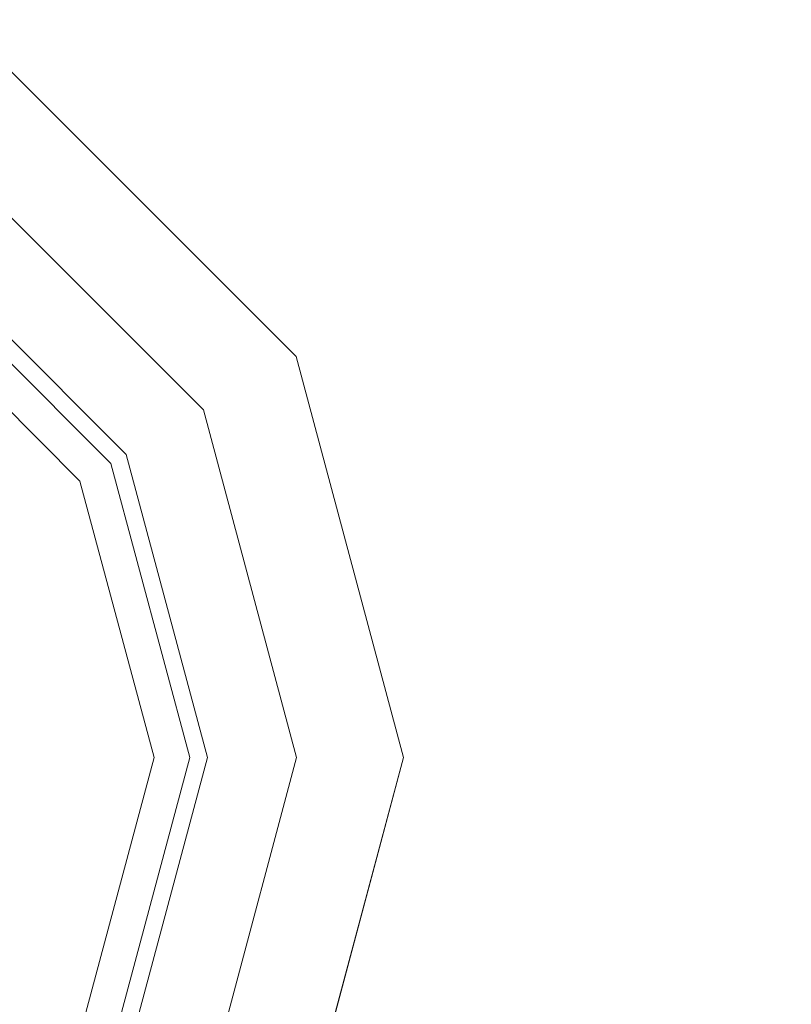
# Model space of a CAD drawing. Units: inches. Extents: x 375 to 1122, y 27 to 1069.
# Tile 123 of 155: x 715.443 to 720.771, y 893.412 to 900.211. Entities that reach past the tile are written whole.
import ezdxf

# ---------------------------------------------------------------- set-up
doc = ezdxf.new("R2010")
doc.units = ezdxf.units.IN
doc.layers.add('A-ANNO-DIMS', color=2, linetype='Continuous', lineweight=18)
doc.layers.add('Furniture', color=30, linetype='Continuous', lineweight=18)
doc.styles.get("Standard").update_dxf_attribs({"font": 'arial.ttf'})
doc.dimstyles.new('ISO-25', dxfattribs={"dimtxt": 12, "dimasz": 2.5, "dimexe": 1.5, "dimexo": 1.5, "dimtad": 1, "dimdec": 1, "dimlunit": 3, "dimtxsty": 'Standard', "dimblk": 'ARCHTICK', "dimcen": 2.5, "dimadec": 0, "dimazin": 0, "dimtfac": 1, "dimtdec": 1, "dimtmove": 0, "dimatfit": 3, "dimfxl": 1.5, "dimfxlon": 1, "dimarcsym": 0})

# ---------------------------------------------------------------- blocks, each defined once
blk = doc.blocks.new('A$C403C54AD')
at = {"linetype": 'ByBlock'}
for points, invisible_edges in [([(1.0802, 0.82864, -0.00874), (1.0802, 0.81017, -0.00874), (1.02018, 0.79408, -0.00874), (1.01094, 0.81008, -0.00874)], 5), ([(1.0802, 0.79478, -0.02259), (1.0802, 0.82864, -0.01335), (1.01094, 0.81008, -0.01335), (1.02787, 0.78075, -0.02259)], 5), ([(1.14947, 0.81008, -0.00874), (1.14023, 0.79408, -0.00874), (1.0802, 0.81017, -0.00874), (1.0802, 0.82864, -0.00874)], 5), ([(1.13254, 0.78075, -0.02259), (1.14947, 0.81008, -0.01335), (1.0802, 0.82864, -0.01335), (1.0802, 0.79478, -0.02259)], 5), ([(1.01094, 0.81008, -0.00874), (1.02018, 0.79408, -0.00874), (0.97623, 0.75014, -0.00874), (0.96024, 0.75938, -0.00874)], 5), ([(1.02787, 0.78075, -0.02259), (1.01094, 0.81008, -0.01335), (0.96024, 0.75938, -0.01335), (0.98956, 0.74244, -0.02259)], 5), ([(1.0802, 0.81017, -0.00874), (1.0802, 0.7917, -0.01489), (1.02941, 0.77809, -0.01489), (1.02018, 0.79408, -0.00874)], 5), ([(1.14023, 0.79408, -0.00874), (1.131, 0.77809, -0.01489), (1.0802, 0.7917, -0.01489), (1.0802, 0.81017, -0.00874)], 5), ([(1.02018, 0.79408, -0.00874), (1.02941, 0.77809, -0.01489), (0.99223, 0.74091, -0.01489), (0.97623, 0.75014, -0.00874)], 5), ([(1.0802, 0.78554, -0.03183), (1.0802, 0.79478, -0.02259), (1.02787, 0.78075, -0.02259), (1.03249, 0.77276, -0.03183)], 5), ([(1.12792, 0.77276, -0.03183), (1.13254, 0.78075, -0.02259), (1.0802, 0.79478, -0.02259), (1.0802, 0.78554, -0.03183)], 5), ([(1.0802, 0.7917, -0.01489), (1.0802, 0.69011, -0.01489), (1.0802, 0.69011, -0.01489), (1.02941, 0.77809, -0.01489)], 5), ([(1.131, 0.77809, -0.01489), (1.0802, 0.69011, -0.01489), (1.0802, 0.69011, -0.01489), (1.0802, 0.7917, -0.01489)], 5), ([(1.03249, 0.77276, -0.03183), (1.02787, 0.78075, -0.02259), (0.98956, 0.74244, -0.02259), (0.99756, 0.73783, -0.03183)], 1), ([(1.02941, 0.77809, -0.01489), (1.0802, 0.69011, -0.01489), (1.0802, 0.69011, -0.01489), (0.99223, 0.74091, -0.01489)], 5), ([(1.16818, 0.74091, -0.01489), (1.0802, 0.69011, -0.01489), (1.0802, 0.69011, -0.01489), (1.131, 0.77809, -0.01489)], 5)]:
    blk.add_3dface(points, dxfattribs=dict(at, invisible_edges=invisible_edges))
for points in [[(1.0802, 0.82864, -0.01335), (1.0802, 0.82864, -0.00874), (1.01094, 0.81008, -0.00874), (1.01094, 0.81008, -0.01335)], [(1.14947, 0.81008, -0.01335), (1.14947, 0.81008, -0.00874), (1.0802, 0.82864, -0.00874), (1.0802, 0.82864, -0.01335)], [(1.01094, 0.81008, -0.01335), (1.01094, 0.81008, -0.00874), (0.96024, 0.75938, -0.00874), (0.96024, 0.75938, -0.01335)]]:
    blk.add_3dface(points, dxfattribs=at)
blk = doc.blocks.new('_ArchTick')
at = {"color": 0, "linetype": 'ByBlock', "const_width": 0.15}
blk.add_lwpolyline([(-0.5, -0.5), (0.5, 0.5)], dxfattribs=at)
blk = doc.blocks.new('*D73')
at = {"layer": 'A-ANNO-DIMS', "color": 0, "lineweight": -2, "transparency": 16777216}
for p, q in [((686.7573, 932.4277), (686.7573, 929.4277)), ((770.7573, 932.4277), (770.7573, 929.4277)), ((686.7573, 930.9277), (770.7573, 930.9277)), ((770.7573, 930.9277), (987.6096, 930.9277))]:
    blk.add_line(p, q, dxfattribs=at)
at = {"layer": 'Defpoints', "color": 0, "transparency": 16777216}
for p in [(686.7573, 943.5277), (770.7573, 943.5277), (770.7573, 930.9277)]:
    blk.add_point(p, dxfattribs=at)
at = {"layer": 'A-ANNO-DIMS', "color": 0, "lineweight": -2, "transparency": 16777216, "xscale": 2.5, "yscale": 2.5, "zscale": 2.5, "rotation": 180}
blk.add_blockref('_ArchTick', (686.7573, 930.9277), dxfattribs=at)
at = {"layer": 'A-ANNO-DIMS', "color": 0, "lineweight": -2, "transparency": 16777216, "xscale": 2.5, "yscale": 2.5, "zscale": 2.5}
blk.add_blockref('_ArchTick', (770.7573, 930.9277), dxfattribs=at)
at = {"layer": 'A-ANNO-DIMS', "color": 0, "transparency": 16777216, "insert": (880.4335, 937.7573), "char_height": 12, "attachment_point": 5}
blk.add_mtext('2-PANEL SLIDER 7\'-0" TYP.', dxfattribs=at)

msp = doc.modelspace()

# ---------------------------------------------------------------- block references
at = {"layer": 'Furniture', "xscale": 39.9918517141215, "yscale": 39.9918517141215, "zscale": 39.9918517141215, "rotation": 270}
msp.add_blockref('A$C403C54AD', (684.9549, 938.3156, 0.024), dxfattribs=at)

# ---------------------------------------------------------------- dimensions: what is measured, and where the dimension line sits
at = {"layer": 'A-ANNO-DIMS'}
dim = msp.add_linear_dim(base=(770.7573, 930.9277), p1=(686.7573, 943.5277), p2=(770.7573, 943.5277), text='2-PANEL SLIDER <> TYP.', dimstyle='ISO-25', override={"dimdec": 1, "dimlfac": 1, "dimrnd": 0, "dimzin": 1, "dimdsep": 46, "dimlunit": 4, "dimfrac": 2}, dxfattribs=at)
dim.commit()
dim.dimension.update_dxf_attribs({"geometry": '*D73', "text_midpoint": (880.4335, 937.7573)})

doc.saveas('drawing.dxf')
